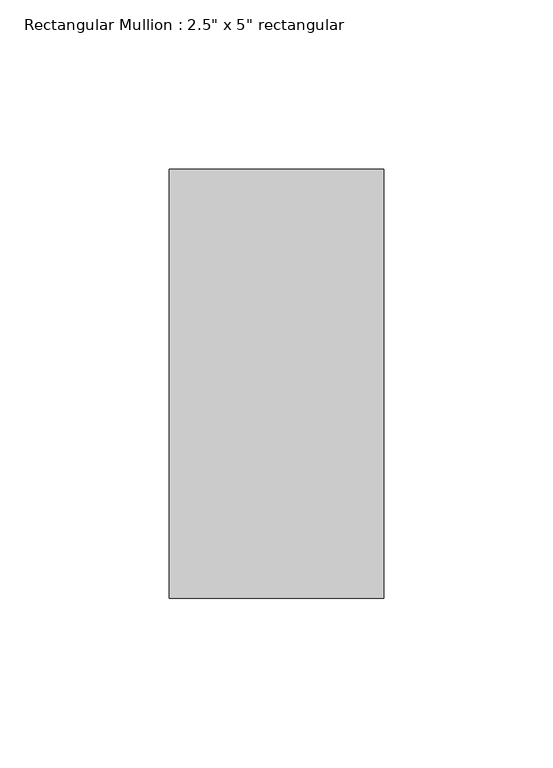
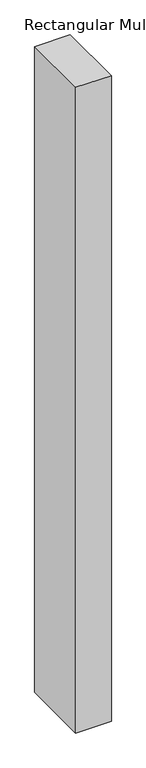
"""IFC4 building model written with IfcOpenShell, lengths in millimetres: member geometry."""

from ifc_helpers import new_model, si_unit, frame, origin, place, context, project, spatial, polyline, outline, extrude, source, transform, mapped, element, save


def member_75074519(model_context):
    return source(origin(), model_context, "Body", "SweptSolid", [
        extrude(outline(polyline([(0.0, 63.5), (0.0, -63.5), (-63.5, -63.5), (-63.5, 63.5), (0.0, 63.5)])), frame((0.0, 0.0, -1219.2), z_axis=(0.0, 0.0, 1.0), x_axis=(1.0, 0.0, 0.0)), (0.0, 0.0, 1.0), 1219.2),
    ])


if __name__ == "__main__":
    model = new_model("IFC4")
    model_context = context("Model", 3, world=origin())
    ifc_project = project(units=[si_unit("LENGTHUNIT", "METRE", prefix="MILLI")], contexts=[model_context])
    site = spatial("IfcSite", under=ifc_project)
    building = spatial("IfcBuilding", under=site)
    placement = place(None, origin())
    member_shape = member_75074519(model_context)
    element("IfcMember", 1, ObjectType="Rectangular Mullion : 2.5\" x 5\" rectangular", at=placement, inside=building, context=model_context, shape_type="MappedRepresentation", body=[
        mapped(member_shape, transform((0.0, 0.0, 0.0), x_axis=(1.0, 0.0, 0.0), y_axis=(0.0, 1.0, 0.0), z_axis=(0.0, 0.0, 1.0))),
    ])
    save(model, "model.ifc")

# Revit data of these elements
# Type "Rectangular Mullion : 2.5\" x 5\" rectangular"
#   built-in parameter 1007304 = 0.416667 (stored number, unit not read)
#   built-in parameter 1007301 = 0.104167 (stored number, unit not read)
#   built-in parameter 1007300 = 0.104167 (stored number, unit not read)
# Element 1 (IfcMember, "Rectangular Mullion : 2.5\" x 5\" rectangular")
#   Materials on its faces: "Iron, Ductile"
# Materials
#   "Iron, Ductile": class "Metal", colour RGB 0 0 0, transparency 0, Description = "Ductile cast iron", Cost = 0
